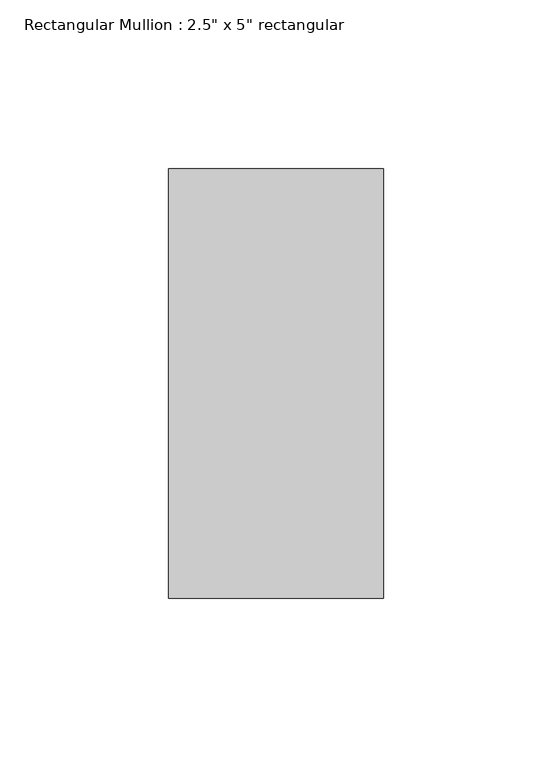
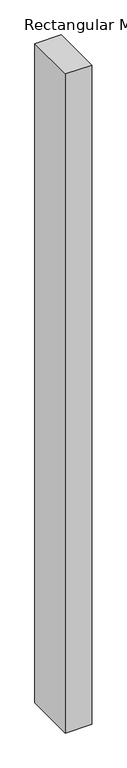
"""IFC4 building model written with IfcOpenShell, lengths in millimetres: member geometry."""

from ifc_helpers import new_model, si_unit, frame, origin, place, context, project, spatial, polyline, outline, extrude, source, transform, mapped, element, save


def member_5e920210(model_context):
    return source(origin(), model_context, "Body", "SweptSolid", [
        extrude(outline(polyline([(31.75, 63.5), (31.75, -63.5), (-31.75, -63.5), (-31.75, 63.5), (31.75, 63.5)])), frame((0.0, 0.0, -1682.0744644), z_axis=(0.0, 0.0, 1.0), x_axis=(1.0, 0.0, 0.0)), (0.0, 0.0, 1.0), 1682.0744644),
    ])


if __name__ == "__main__":
    model = new_model("IFC4")
    model_context = context("Model", 3, world=origin())
    ifc_project = project(units=[si_unit("LENGTHUNIT", "METRE", prefix="MILLI")], contexts=[model_context])
    site = spatial("IfcSite", under=ifc_project)
    building = spatial("IfcBuilding", under=site)
    placement = place(None, origin())
    member_shape = member_5e920210(model_context)
    element("IfcMember", 1, ObjectType="Rectangular Mullion : 2.5\" x 5\" rectangular", at=placement, inside=building, context=model_context, shape_type="MappedRepresentation", body=[
        mapped(member_shape, transform((0.0, 0.0, 0.0), x_axis=(1.0, 0.0, 0.0), y_axis=(0.0, 1.0, 0.0), z_axis=(0.0, 0.0, 1.0))),
    ])
    save(model, "model.ifc")

# Revit data of these elements
# Type "Rectangular Mullion : 2.5\" x 5\" rectangular"
#   built-in parameter 1007304 = 0.416667 (stored number, unit not read)
#   built-in parameter 1007301 = 0.104167 (stored number, unit not read)
#   built-in parameter 1007300 = 0.104167 (stored number, unit not read)
# Element 1 (IfcMember, "Rectangular Mullion : 2.5\" x 5\" rectangular")
#   Materials on its faces: "Aluminum"
# Materials
#   "Aluminum": class "Metal", colour RGB 247 247 247, transparency 0, Description = "Aluminum 6061", Cost = 0
